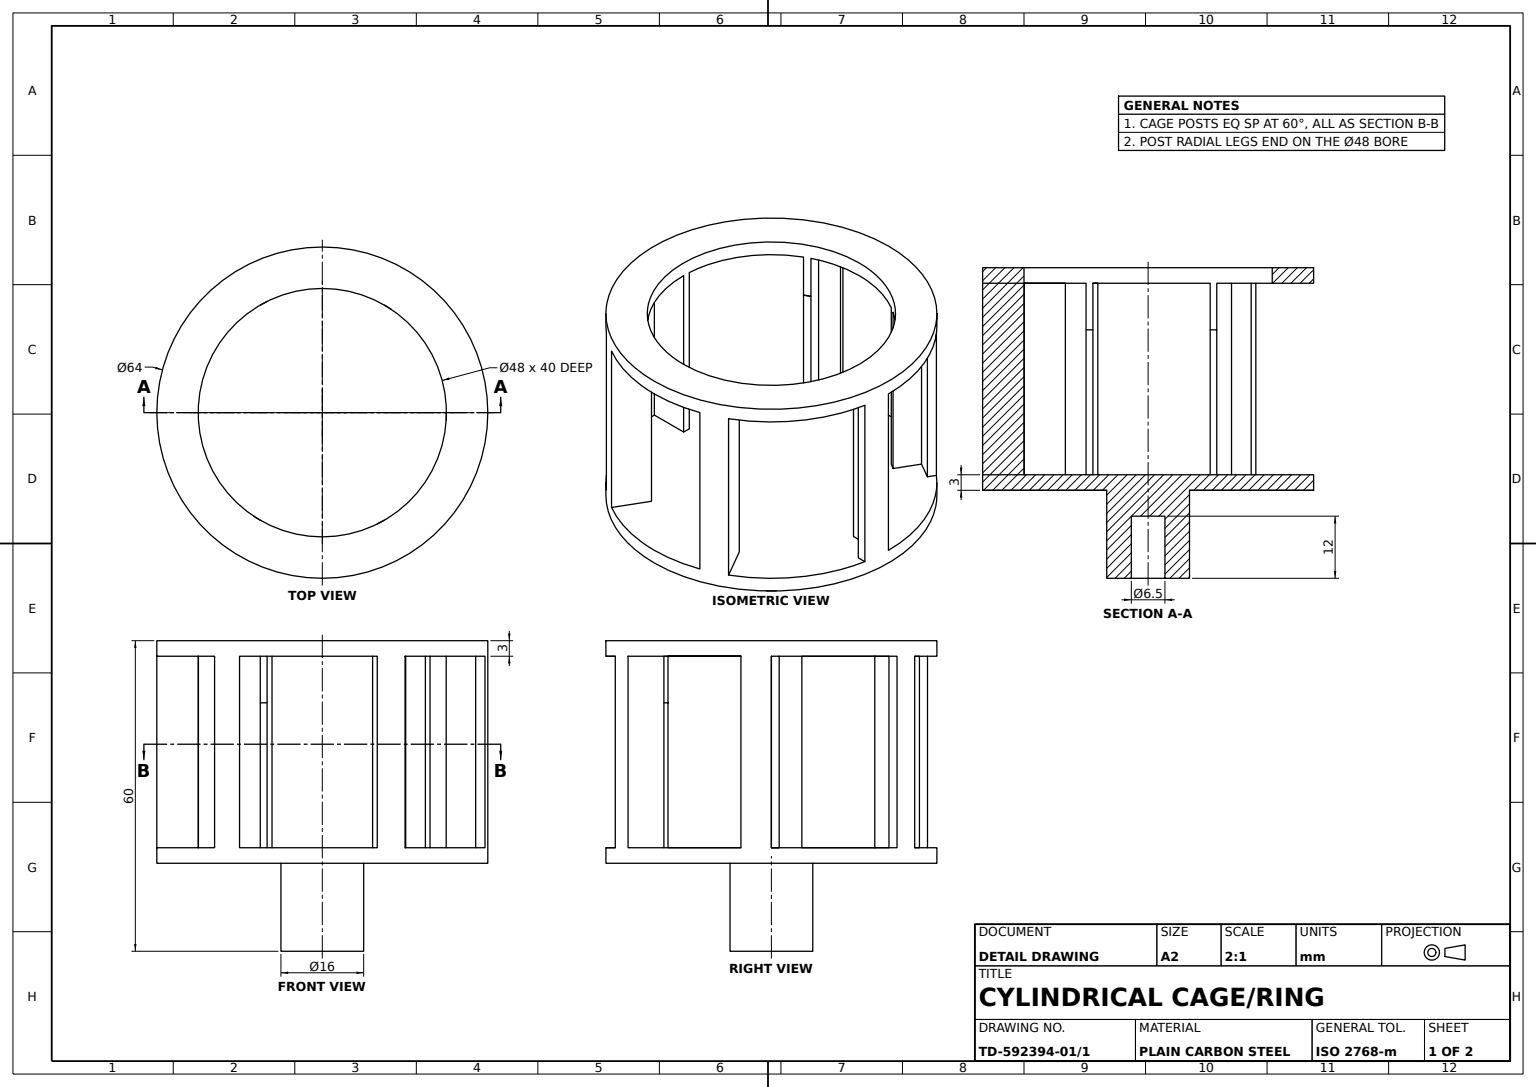
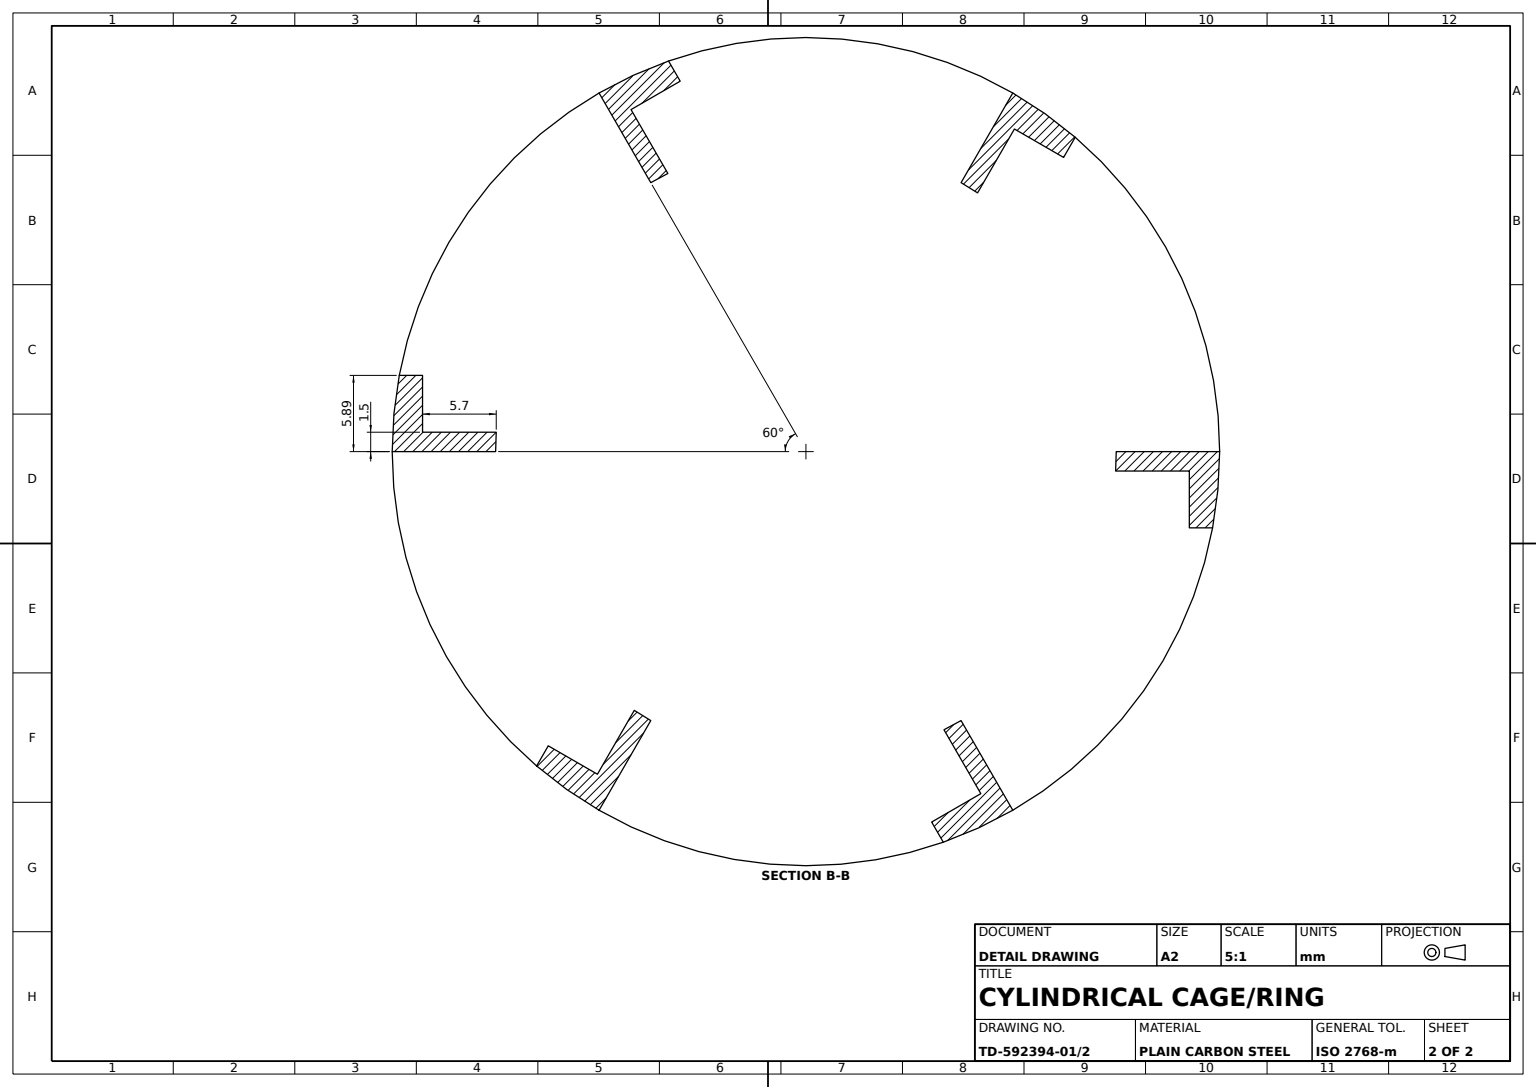
from build123d import *
from build123d.topology import SkipClean

# Parameters (mm, degrees)
BASE_DISC_SKETCH_R    = 32
BASE_DISC_64_DEPTH    = 3
CAGE_POSTS_6X_DEPTH   = 40
TOP_START             = -3
TOP_RING_SKETCH_R     = 32
TOP_RING_DEPTH        = 3
HUB_SKETCH_R          = 8
HUB_16_DEPTH          = 17
HUB_BORE_SKETCH_R     = 3.25
HUB_BORE_6_5_DEPTH    = 12
INNER_START           = -12
INNER_RECESS_SKETCH_R = 24
INNER_RECESS_48_DEPTH = 12


with BuildPart() as part:
    # Base Disc Sketch → Base Disc Ø64 (new body)
    with BuildSketch(Plane(origin=(0, 0, 0), x_dir=(1, 0, 0), z_dir=(0, 1, 0))):
        with Locations(Location((0, 0, 0), (0, 0, 270))):
            Circle(BASE_DISC_SKETCH_R)
    extrude(amount=BASE_DISC_64_DEPTH)

    # Cage Posts Sketch → Cage Posts 6x (add)
    with SkipClean():  # the faces are left unmerged after this step: merging them gives an invalid solid
        with BuildSketch(Plane(origin=(0, 3, 0), x_dir=(1, 0, 0), z_dir=(0, 1, 0))):
            with BuildLine():
                Line((-19.928290222, -22.734822717), (-20.828290222, -24.293668443))
                ThreePointArc((-20.828290222, -24.293668443), (-18.493333323, -26.115065051), (-16, -27.712812921))
                Line((-16, -27.712812921), (-12, -20.784609691))
                Line((-12, -20.784609691), (-13.275577673, -19.993975029))
                Line((-13.275577673, -19.993975029), (-16.125577673, -24.93031983))
                Line((-16.125577673, -24.93031983), (-19.928290222, -22.734822717))
            make_face()
            with BuildLine():
                Line((29.653079134, -5.890994228), (31.453079134, -5.890994228))
                ThreePointArc((31.453079134, -5.890994228), (31.862976417, -2.958163933), (32, 0))
                Line((32, 0), (24, 0))
                Line((24, 0), (23.953079134, -1.5))
                Line((23.953079134, -1.5), (29.653079134, -1.5))
                Line((29.653079134, -1.5), (29.653079134, -5.890994228))
            make_face()
            with BuildLine():
                ThreePointArc((20.828290222, 24.293668443), (18.493333323, 26.115065051), (16, 27.712812921))
                Line((16, 27.712812921), (12, 20.784609691))
                Line((12, 20.784609691), (13.275577673, 19.993975029))
                Line((13.275577673, 19.993975029), (16.125577673, 24.93031983))
                Line((16.125577673, 24.93031983), (19.928290222, 22.734822717))
                Line((19.928290222, 22.734822717), (20.828290222, 24.293668443))
            make_face()
            with BuildLine():
                Line((-32, 0), (-24, 0))
                ThreePointArc((-24, 0), (-23.988266915, 0.750366838), (-23.953079134, 1.5))
                Line((-23.953079134, 1.5), (-29.653079134, 1.5))
                Line((-29.653079134, 1.5), (-29.653079134, 5.890994228))
                Line((-29.653079134, 5.890994228), (-31.453079134, 5.890994228))
                ThreePointArc((-31.453079134, 5.890994228), (-31.862976417, 2.958163933), (-32, 0))
            make_face()
            with BuildLine():
                Line((9.724788912, -28.625816944), (13.527501461, -26.43031983))
                Line((13.527501461, -26.43031983), (10.677501461, -21.493975029))
                Line((10.677501461, -21.493975029), (12, -20.784609691))
                Line((12, -20.784609691), (16, -27.712812921))
                ThreePointArc((16, -27.712812921), (13.369643094, -29.073228984), (10.624788912, -30.184662671))
                Line((10.624788912, -30.184662671), (9.724788912, -28.625816944))
            make_face()
            with BuildLine():
                ThreePointArc((-16, 27.712812921), (-13.369643094, 29.073228984), (-10.624788912, 30.184662671))
                Line((-10.624788912, 30.184662671), (-9.724788912, 28.625816944))
                Line((-9.724788912, 28.625816944), (-13.527501461, 26.43031983))
                Line((-13.527501461, 26.43031983), (-10.677501461, 21.493975029))
                Line((-10.677501461, 21.493975029), (-12, 20.784609691))
                Line((-12, 20.784609691), (-16, 27.712812921))
            make_face()
        extrude(amount=CAGE_POSTS_6X_DEPTH)

    # Top Ring Sketch → Top Ring (add)
    with SkipClean():  # the faces are left unmerged after this step: merging them gives an invalid solid
        with BuildSketch(Plane(origin=(0, 43, 0), x_dir=(1, 0, 0), z_dir=(0, 1, 0)).offset(TOP_START)):
            with Locations(Location((0, 0, 0), (0, 0, 270))):
                Circle(TOP_RING_SKETCH_R)
        extrude(amount=TOP_RING_DEPTH)

    # Hub Sketch → Hub Ø16 (add)
    with SkipClean():  # the faces are left unmerged after this step: merging them gives an invalid solid
        with BuildSketch(Plane.XZ):
            with Locations(Location((0, 0, 0), (0, 0, 270))):
                Circle(HUB_SKETCH_R)
        extrude(amount=HUB_16_DEPTH)

    # Hub Bore Sketch → Hub Bore Ø6.5 (cut)
    with SkipClean():  # the faces are left unmerged after this step: merging them gives an invalid solid
        with BuildSketch(Plane.XZ.offset(17)):
            with Locations(Location((0, 0, 0), (0, 0, 270))):
                Circle(HUB_BORE_SKETCH_R)
        extrude(amount=-HUB_BORE_6_5_DEPTH, mode=Mode.SUBTRACT)

    # Inner Recess Sketch → Inner Recess Ø48 (cut)
    with SkipClean():  # the faces are left unmerged after this step: merging them gives an invalid solid
        with BuildSketch(Plane(origin=(0, 43, 0), x_dir=(1, 0, 0), z_dir=(0, 1, 0)).offset(INNER_START)):
            with Locations(Location((0, 0, 0), (0, 0, 116.416678302))):
                Circle(INNER_RECESS_SKETCH_R)
        extrude(amount=INNER_RECESS_48_DEPTH, mode=Mode.SUBTRACT)


solid = part.part
